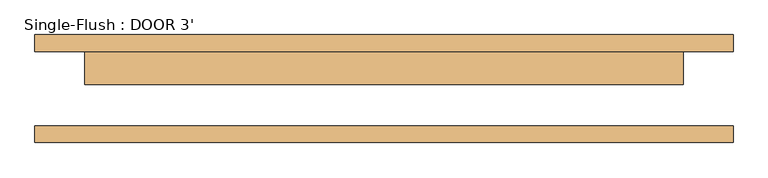
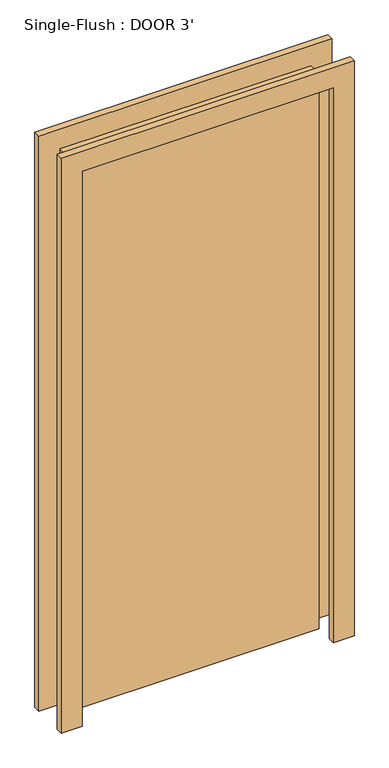
"""IFC4 building model written with IfcOpenShell, lengths in millimetres: door geometry, Single-Flush : DOOR 3'."""

from ifc_helpers import new_model, si_unit, frame, origin, origin_with_axes, place, context, project, spatial, polyline, outline, extrude, source, transform, mapped, element, save


def single_flush_door_3_e5f9f3c4(model_context):
    return source(origin(), model_context, "Body", "SweptSolid", [
        extrude(outline(polyline([(2209.8, -533.4), (0.0, -533.4), (0.0, -457.2), (2133.6, -457.2), (2133.6, 457.2), (0.0, 457.2), (0.0, 533.4), (2209.8, 533.4), (2209.8, -533.4)])), frame((0.0, 57.15, 0.0), z_axis=(0.0, 1.0, 0.0), x_axis=(0.0, 0.0, 1.0)), (0.0, 0.0, 1.0), 25.4),
        extrude(outline(polyline([(2209.8, 533.4), (2209.8, -533.4), (0.0, -533.4), (0.0, -457.2), (2133.6, -457.2), (2133.6, 457.2), (0.0, 457.2), (0.0, 533.4), (2209.8, 533.4)])), frame((0.0, -82.55, 0.0), z_axis=(0.0, 1.0, 0.0), x_axis=(0.0, 0.0, 1.0)), (0.0, 0.0, 1.0), 25.4),
        extrude(outline(polyline([(457.2, 6.35), (-457.2, 6.35), (-457.2, 57.15), (457.2, 57.15), (457.2, 6.35)])), origin_with_axes(), (0.0, 0.0, 1.0), 2133.6),
    ])


if __name__ == "__main__":
    model = new_model("IFC4")
    model_context = context("Model", 3, world=origin())
    ifc_project = project(units=[si_unit("LENGTHUNIT", "METRE", prefix="MILLI")], contexts=[model_context])
    site = spatial("IfcSite", under=ifc_project)
    building = spatial("IfcBuilding", under=site)
    placement = place(None, origin())
    single_flush_door_3_shape = single_flush_door_3_e5f9f3c4(model_context)
    element("IfcDoor", 1, ObjectType="Single-Flush : DOOR 3'", at=placement, inside=building, context=model_context, shape_type="MappedRepresentation", body=[
        mapped(single_flush_door_3_shape, transform((0.0, 0.0, 0.0), x_axis=(1.0, 0.0, 0.0), y_axis=(0.0, 1.0, 0.0), z_axis=(0.0, 0.0, 1.0))),
    ])
    save(model, "model.ifc")

# Revit data of these elements
# Type "Single-Flush : DOOR 3'"
#   Type Mark = "8"
#   Construction Type Id = "MDOOR"
#   Assembly Code = "C1020"
#   Analytic Construction = "Metal"
#   Thickness = 0' - 2"
#   Heat Transfer Coefficient (U) = 0.651978 BTU/(h·ft²·°F)
#   Height = 7' - 0"
#   Trim Projection Ext = 0' - 1"
#   Trim Projection Int = 0' - 1"
#   Trim Width = 0' - 3"
#   Width = 3' - 0"
#   Define Thermal Properties by = 1
#   Door Material = Door - Panel
#   Frame Material = Door - Frame
#   Visual Light Transmittance = 0
#   Solar Heat Gain Coefficient = 0
#   Function = (empty or 0)
#   Wall Closure = (empty or 0)
# Element 1 (IfcDoor, "Single-Flush : DOOR 3'")
#   Materials on its faces: "Door - Frame", "Door - Panel"
# Materials
#   "Door - Panel": class "Wood", colour RGB 210 159 95, transparency 0, Cost = 0
#   "Door - Frame": colour RGB 118 70 51, transparency 0, Cost = 0
